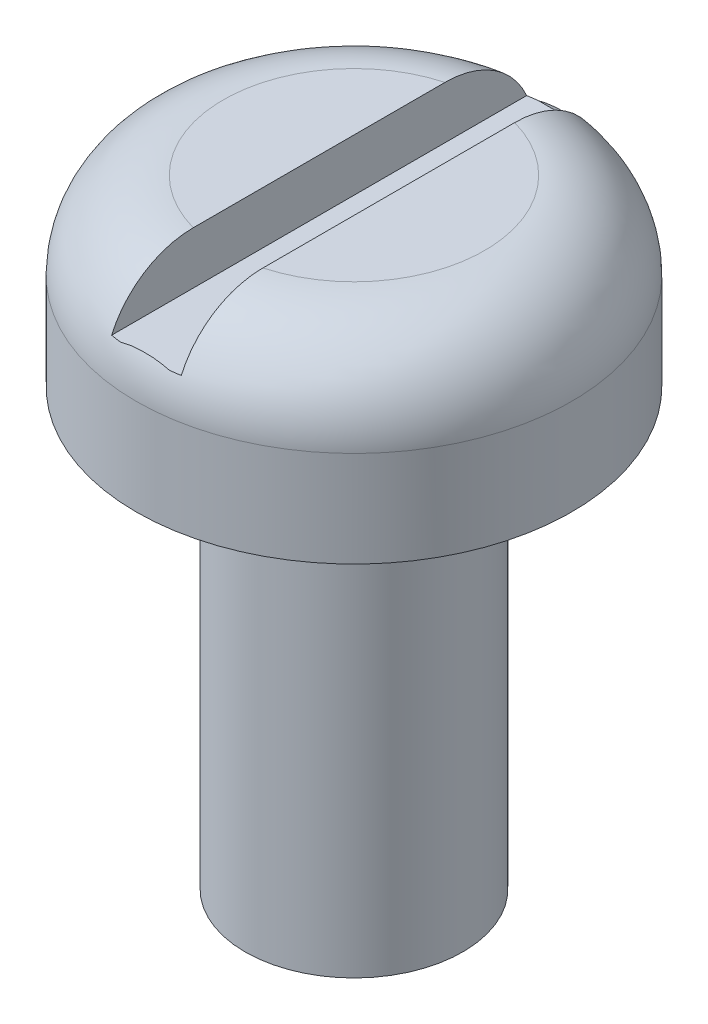
ISO-10303-21;
HEADER;
FILE_DESCRIPTION(('STEP AP214'),'2;1');
FILE_NAME('part.step','',(''),(''),'','','');
FILE_SCHEMA(('AUTOMOTIVE_DESIGN { 1 0 10303 214 1 1 1 1 }'));
ENDSEC;
DATA;
#1=APPLICATION_CONTEXT('core data for automotive mechanical design processes');
#2=APPLICATION_PROTOCOL_DEFINITION('international standard','automotive_design',2000,#1);
#3=PRODUCT_CONTEXT('',#1,'mechanical');
#4=PRODUCT('Part','Part','',(#3));
#5=PRODUCT_RELATED_PRODUCT_CATEGORY('part','',(#4));
#6=PRODUCT_DEFINITION_FORMATION('','',#4);
#7=PRODUCT_DEFINITION_CONTEXT('part definition',#1,'design');
#8=PRODUCT_DEFINITION('design','',#6,#7);
#9=PRODUCT_DEFINITION_SHAPE('','',#8);
#10=(LENGTH_UNIT() NAMED_UNIT(*) SI_UNIT(.MILLI.,.METRE.));
#11=(NAMED_UNIT(*) PLANE_ANGLE_UNIT() SI_UNIT($,.RADIAN.));
#12=(NAMED_UNIT(*) SI_UNIT($,.STERADIAN.) SOLID_ANGLE_UNIT());
#13=UNCERTAINTY_MEASURE_WITH_UNIT(LENGTH_MEASURE(1.E-05),#10,'distance_accuracy_value','');
#14=(GEOMETRIC_REPRESENTATION_CONTEXT(3) GLOBAL_UNCERTAINTY_ASSIGNED_CONTEXT((#13)) GLOBAL_UNIT_ASSIGNED_CONTEXT((#10,
#11,#12)) REPRESENTATION_CONTEXT('',''));
#15=CARTESIAN_POINT('',(0.,0.,0.));
#16=DIRECTION('',(0.,0.,1.));
#17=DIRECTION('',(1.,0.,0.));
#18=AXIS2_PLACEMENT_3D('',#15,#16,#17);
#19=CARTESIAN_POINT('',(0.,2.1,0.));
#20=DIRECTION('',(0.,-1.,0.));
#21=DIRECTION('',(0.,0.,-1.));
#22=AXIS2_PLACEMENT_3D('',#19,#20,#21);
#23=PLANE('',#22);
#24=CARTESIAN_POINT('',(0.,2.1,0.));
#25=DIRECTION('',(0.,-1.,0.));
#26=DIRECTION('',(0.,0.,-1.));
#27=AXIS2_PLACEMENT_3D('',#24,#25,#26);
#28=CIRCLE('',#27,1.5);
#29=CARTESIAN_POINT('',(0.4,2.1,1.4456832294801));
#30=VERTEX_POINT('',#29);
#31=CARTESIAN_POINT('',(0.4,2.1,-1.4456832294801));
#32=VERTEX_POINT('',#31);
#33=EDGE_CURVE('E110',#30,#32,#28,.F.);
#34=ORIENTED_EDGE('',*,*,#33,.T.);
#35=DIRECTION('',(0.,0.,-1.));
#36=VECTOR('',#35,1.);
#37=CARTESIAN_POINT('',(0.4,2.1,2.4));
#38=LINE('',#37,#36);
#39=EDGE_CURVE('E97',#30,#32,#38,.T.);
#40=ORIENTED_EDGE('',*,*,#39,.F.);
#41=EDGE_LOOP('',(#34,#40));
#42=FACE_BOUND('',#41,.T.);
#43=ADVANCED_FACE('F39',(#42),#23,.F.);
#44=CARTESIAN_POINT('',(0.,-5.,0.));
#45=DIRECTION('',(0.,1.,0.));
#46=DIRECTION('',(0.,0.,1.));
#47=AXIS2_PLACEMENT_3D('',#44,#45,#46);
#48=PLANE('',#47);
#49=CARTESIAN_POINT('',(0.,-5.,0.));
#50=DIRECTION('',(0.,1.,0.));
#51=DIRECTION('',(0.,0.,1.));
#52=AXIS2_PLACEMENT_3D('',#49,#50,#51);
#53=CIRCLE('',#52,1.25);
#54=CARTESIAN_POINT('',(0.,-5.,1.25));
#55=VERTEX_POINT('',#54);
#56=EDGE_CURVE('E113',#55,#55,#53,.T.);
#57=ORIENTED_EDGE('',*,*,#56,.F.);
#58=EDGE_LOOP('',(#57));
#59=FACE_BOUND('',#58,.T.);
#60=ADVANCED_FACE('F172',(#59),#48,.F.);
#61=CARTESIAN_POINT('',(0.,4.11096256684492,0.));
#62=DIRECTION('',(0.,1.,0.));
#63=DIRECTION('',(0.,0.,1.));
#64=AXIS2_PLACEMENT_3D('',#61,#62,#63);
#65=CYLINDRICAL_SURFACE('',#64,1.25);
#66=CARTESIAN_POINT('',(0.,0.,0.));
#67=DIRECTION('',(0.,1.,0.));
#68=DIRECTION('',(0.,0.,1.));
#69=AXIS2_PLACEMENT_3D('',#66,#67,#68);
#70=CIRCLE('',#69,1.25);
#71=CARTESIAN_POINT('',(0.,0.,1.25));
#72=VERTEX_POINT('',#71);
#73=EDGE_CURVE('E116',#72,#72,#70,.T.);
#74=ORIENTED_EDGE('',*,*,#73,.F.);
#75=EDGE_LOOP('',(#74));
#76=FACE_BOUND('',#75,.T.);
#77=ORIENTED_EDGE('',*,*,#56,.T.);
#78=EDGE_LOOP('',(#77));
#79=FACE_BOUND('',#78,.T.);
#80=ADVANCED_FACE('F180',(#76,#79),#65,.T.);
#81=CARTESIAN_POINT('',(1.25,0.,0.));
#82=DIRECTION('',(0.,1.,0.));
#83=DIRECTION('',(0.,0.,1.));
#84=AXIS2_PLACEMENT_3D('',#81,#82,#83);
#85=PLANE('',#84);
#86=CARTESIAN_POINT('',(0.,0.,0.));
#87=DIRECTION('',(0.,1.,0.));
#88=DIRECTION('',(0.,0.,1.));
#89=AXIS2_PLACEMENT_3D('',#86,#87,#88);
#90=CIRCLE('',#89,2.5);
#91=CARTESIAN_POINT('',(0.,0.,2.5));
#92=VERTEX_POINT('',#91);
#93=EDGE_CURVE('E201',#92,#92,#90,.T.);
#94=ORIENTED_EDGE('',*,*,#93,.F.);
#95=EDGE_LOOP('',(#94));
#96=FACE_BOUND('',#95,.T.);
#97=ORIENTED_EDGE('',*,*,#73,.T.);
#98=EDGE_LOOP('',(#97));
#99=FACE_BOUND('',#98,.T.);
#100=ADVANCED_FACE('F188',(#96,#99),#85,.F.);
#101=CARTESIAN_POINT('',(0.,4.11096256684492,0.));
#102=DIRECTION('',(0.,1.,0.));
#103=DIRECTION('',(0.,0.,1.));
#104=AXIS2_PLACEMENT_3D('',#101,#102,#103);
#105=CYLINDRICAL_SURFACE('',#104,2.5);
#106=CARTESIAN_POINT('',(0.,1.1,0.));
#107=DIRECTION('',(0.,-1.,0.));
#108=DIRECTION('',(0.,0.,-1.));
#109=AXIS2_PLACEMENT_3D('',#106,#107,#108);
#110=CIRCLE('',#109,2.5);
#111=CARTESIAN_POINT('',(0.,1.1,-2.5));
#112=VERTEX_POINT('',#111);
#113=EDGE_CURVE('E117',#112,#112,#110,.T.);
#114=ORIENTED_EDGE('',*,*,#113,.T.);
#115=EDGE_LOOP('',(#114));
#116=FACE_BOUND('',#115,.T.);
#117=ORIENTED_EDGE('',*,*,#93,.T.);
#118=EDGE_LOOP('',(#117));
#119=FACE_BOUND('',#118,.T.);
#120=ADVANCED_FACE('F182',(#116,#119),#105,.T.);
#121=CARTESIAN_POINT('',(-0.4,2.1,-1.4456832294801));
#122=VERTEX_POINT('',#121);
#123=CARTESIAN_POINT('',(-0.4,2.1,1.4456832294801));
#124=VERTEX_POINT('',#123);
#125=EDGE_CURVE('E111',#122,#124,#28,.F.);
#126=ORIENTED_EDGE('',*,*,#125,.T.);
#127=DIRECTION('',(0.,0.,1.));
#128=VECTOR('',#127,1.);
#129=CARTESIAN_POINT('',(-0.4,2.1,2.4));
#130=LINE('',#129,#128);
#131=EDGE_CURVE('E107',#122,#124,#130,.T.);
#132=ORIENTED_EDGE('',*,*,#131,.F.);
#133=EDGE_LOOP('',(#126,#132));
#134=FACE_BOUND('',#133,.T.);
#135=ADVANCED_FACE('F147',(#134),#23,.F.);
#136=CARTESIAN_POINT('',(0.,1.1,0.));
#137=DIRECTION('',(0.,-1.,0.));
#138=DIRECTION('',(0.,0.,-1.));
#139=AXIS2_PLACEMENT_3D('',#136,#137,#138);
#140=TOROIDAL_SURFACE('',#139,1.5,1.);
#141=CARTESIAN_POINT('',(-0.4,1.37314136652749,0.359822287950911));
#142=CARTESIAN_POINT('',(-0.4,1.40093270642667,0.371622303440927));
#143=CARTESIAN_POINT('',(-0.4,1.42812821348821,0.384783955279465));
#144=CARTESIAN_POINT('',(-0.4,1.48131846126341,0.413357432969681));
#145=CARTESIAN_POINT('',(-0.4,1.50731251310842,0.428770529152034));
#146=CARTESIAN_POINT('',(-0.4,1.58346389369532,0.477895994599856));
#147=CARTESIAN_POINT('',(-0.4,1.63178371791217,0.514491510849547));
#148=CARTESIAN_POINT('',(-0.4,1.72575940533382,0.596458724839461));
#149=CARTESIAN_POINT('',(-0.4,1.77105848354616,0.642236723330395));
#150=CARTESIAN_POINT('',(-0.4,1.85432920614574,0.739995997687899));
#151=CARTESIAN_POINT('',(-0.4,1.89230615268545,0.791972740397109));
#152=CARTESIAN_POINT('',(-0.4,1.96395225809638,0.908108851081128));
#153=CARTESIAN_POINT('',(-0.4,1.99648409188238,0.972978581679796));
#154=CARTESIAN_POINT('',(-0.4,2.04899259975919,1.10766848251091));
#155=CARTESIAN_POINT('',(-0.4,2.06896827937325,1.17748904437354));
#156=CARTESIAN_POINT('',(-0.4,2.0938680591257,1.31338506858809));
#157=CARTESIAN_POINT('',(-0.4,2.09996775846476,1.37924512842784));
#158=CARTESIAN_POINT('',(-0.4,2.10003193371477,1.51096708389506));
#159=CARTESIAN_POINT('',(-0.4,2.09400361962018,1.57682895516902));
#160=CARTESIAN_POINT('',(-0.4,2.07067030458484,1.70123764081731));
#161=CARTESIAN_POINT('',(-0.4,2.05427474028281,1.75995595824222));
#162=CARTESIAN_POINT('',(-0.4,2.01140744039179,1.8735942289021));
#163=CARTESIAN_POINT('',(-0.4,1.98493845444247,1.92851521382656));
#164=CARTESIAN_POINT('',(-0.4,1.92400229725042,2.03046814640842));
#165=CARTESIAN_POINT('',(-0.4,1.88993659917133,2.07774038262831));
#166=CARTESIAN_POINT('',(-0.4,1.81417105020338,2.16571110461842));
#167=CARTESIAN_POINT('',(-0.4,1.77247236837605,2.20641059527067));
#168=CARTESIAN_POINT('',(-0.4,1.68373611156411,2.27906555988676));
#169=CARTESIAN_POINT('',(-0.4,1.63685221089368,2.31120885230998));
#170=CARTESIAN_POINT('',(-0.4,1.53829665012664,2.36704528781166));
#171=CARTESIAN_POINT('',(-0.4,1.48662538258074,2.39073912295086));
#172=CARTESIAN_POINT('',(-0.4,1.38069618244624,2.4287008656164));
#173=CARTESIAN_POINT('',(-0.4,1.32648106473839,2.44308832578949));
#174=CARTESIAN_POINT('',(-0.4,1.21639976672113,2.4624969216675));
#175=CARTESIAN_POINT('',(-0.4,1.16053365428317,2.46751844185828));
#176=CARTESIAN_POINT('',(-0.4,1.04908863796257,2.46804320743455));
#177=CARTESIAN_POINT('',(-0.4,0.993509988965319,2.46360255553827));
#178=CARTESIAN_POINT('',(-0.4,0.883889082008193,2.4454495710633));
#179=CARTESIAN_POINT('',(-0.4,0.829846804146247,2.43173735864504));
#180=CARTESIAN_POINT('',(-0.4,0.724842061024363,2.39545342961124));
#181=CARTESIAN_POINT('',(-0.4,0.673878716366111,2.37288425663857));
#182=CARTESIAN_POINT('',(-0.4,0.576438813198237,2.31955230734661));
#183=CARTESIAN_POINT('',(-0.4,0.529962302699139,2.28878944336552));
#184=CARTESIAN_POINT('',(-0.4,0.442543206150293,2.2197899814353));
#185=CARTESIAN_POINT('',(-0.4,0.401630600296936,2.18151541483789));
#186=CARTESIAN_POINT('',(-0.4,0.32672353206193,2.0987119502436));
#187=CARTESIAN_POINT('',(-0.4,0.292729339220681,2.05418280868355));
#188=CARTESIAN_POINT('',(-0.4,0.232169698703393,1.95958819897401));
#189=CARTESIAN_POINT('',(-0.4,0.205696783523953,1.90946352616052));
#190=CARTESIAN_POINT('',(-0.4,0.161349431874205,1.80555086102151));
#191=CARTESIAN_POINT('',(-0.4,0.143475492699256,1.75176265703223));
#192=CARTESIAN_POINT('',(-0.4,0.11638434181792,1.64084211977878));
#193=CARTESIAN_POINT('',(-0.4,0.107358832247017,1.58366304903687));
#194=CARTESIAN_POINT('',(-0.4,0.0986849300413458,1.46860383693886));
#195=CARTESIAN_POINT('',(-0.4,0.0990380349972624,1.41072358509211));
#196=CARTESIAN_POINT('',(-0.4,0.109055349478419,1.29367665174019));
#197=CARTESIAN_POINT('',(-0.4,0.119055025193746,1.23453889656783));
#198=CARTESIAN_POINT('',(-0.4,0.148276458995809,1.11861077758735));
#199=CARTESIAN_POINT('',(-0.4,0.167498607758144,1.06182051333261));
#200=CARTESIAN_POINT('',(-0.4,0.215744233840994,0.948547956472629));
#201=CARTESIAN_POINT('',(-0.4,0.245283691181516,0.892285842264092));
#202=CARTESIAN_POINT('',(-0.4,0.3126427582318,0.784941269175456));
#203=CARTESIAN_POINT('',(-0.4,0.350469724634658,0.733863471656097));
#204=CARTESIAN_POINT('',(-0.4,0.436996253406748,0.633386518111079));
#205=CARTESIAN_POINT('',(-0.4,0.486373171812133,0.584566395985288));
#206=CARTESIAN_POINT('',(-0.4,0.565722481216896,0.517693556759759));
#207=CARTESIAN_POINT('',(-0.4,0.593069815311135,0.496451989280449));
#208=CARTESIAN_POINT('',(-0.4,0.649432632497327,0.456320362883837));
#209=CARTESIAN_POINT('',(-0.4,0.678447348158725,0.437429234624265));
#210=CARTESIAN_POINT('',(-0.4,0.745585160405143,0.397942522412036));
#211=CARTESIAN_POINT('',(-0.4,0.784165027026359,0.378111384529633));
#212=CARTESIAN_POINT('',(-0.4,0.86367896280017,0.344038828478993));
#213=CARTESIAN_POINT('',(-0.4,0.904606064923999,0.329781759484785));
#214=CARTESIAN_POINT('',(-0.4,0.980825865665075,0.310823745651696));
#215=CARTESIAN_POINT('',(-0.4,1.01579220394159,0.304857656892121));
#216=CARTESIAN_POINT('',(-0.4,1.08620228902251,0.299138358795534));
#217=CARTESIAN_POINT('',(-0.4,1.12164512863084,0.299374661447218));
#218=CARTESIAN_POINT('',(-0.4,1.19399937284863,0.306183841661282));
#219=CARTESIAN_POINT('',(-0.4,1.23087368500297,0.313130592971764));
#220=CARTESIAN_POINT('',(-0.4,1.30318937641905,0.332611747138802));
#221=CARTESIAN_POINT('',(-0.4,1.33862491613106,0.345166835899453));
#222=CARTESIAN_POINT('',(-0.4,1.37314136652749,0.359822287950911));
#223=B_SPLINE_CURVE_WITH_KNOTS('',3,(#141,#142,#143,#144,#145,#146,#147,#148,#149,#150,#151,
#152,#153,#154,#155,#156,#157,#158,#159,#160,#161,#162,#163,#164,#165,#166,#167,#168,#169,#170,
#171,#172,#173,#174,#175,#176,#177,#178,#179,#180,#181,#182,#183,#184,#185,#186,#187,#188,#189,
#190,#191,#192,#193,#194,#195,#196,#197,#198,#199,#200,#201,#202,#203,#204,#205,#206,#207,#208,
#209,#210,#211,#212,#213,#214,#215,#216,#217,#218,#219,#220,#221,#222),.UNSPECIFIED.,.T.,.F.,(4,
2,2,2,2,2,2,2,2,2,2,2,2,2,2,2,2,2,2,2,2,2,2,2,2,2,2,2,2,2,2,2,2,2,2,2,2,2,2,2,4),(0.,
0.0905235289434078,0.181098332620318,0.362269841007183,0.554796553029223,0.747183323320209,
0.963694489865064,1.18022280244035,1.37758856742685,1.57483703491976,1.75681028240803,
1.93873389409044,2.11268266628051,2.28660481887703,2.45631680998708,2.62601489748268,
2.79348725921426,2.96095274580354,3.12742806687218,3.29390123044403,3.46032661930264,
3.6267537887674,3.79404491531046,3.96134255824518,4.13061715773694,4.29990154552868,
4.47277739199613,4.64568084369387,4.82482230181395,5.00397134926242,5.19380008899763,
5.38379802447056,5.59114286201002,5.69493236376326,5.79867447202674,5.92848389712762,
6.05792618089144,6.16386383384293,6.26962236175429,6.38163469773545,6.49406363811112),.UNSPECIFIED.);
#224=CARTESIAN_POINT('',(-0.4,1.5,2.38317968625396));
#225=VERTEX_POINT('',#224);
#226=EDGE_CURVE('E11',#124,#225,#223,.T.);
#227=ORIENTED_EDGE('',*,*,#226,.F.);
#228=ORIENTED_EDGE('',*,*,#125,.F.);
#229=CARTESIAN_POINT('',(-0.4,1.8398346166564,-2.13565237677622));
#230=CARTESIAN_POINT('',(-0.4,1.87811511422596,-2.09282132200416));
#231=CARTESIAN_POINT('',(-0.4,1.91273739539628,-2.04667706943084));
#232=CARTESIAN_POINT('',(-0.4,1.9736981507183,-1.94917085805161));
#233=CARTESIAN_POINT('',(-0.4,2.00002839113024,-1.89780377965601));
#234=CARTESIAN_POINT('',(-0.4,2.04370446904179,-1.79147021841471));
#235=CARTESIAN_POINT('',(-0.4,2.06106288392302,-1.73650889676743));
#236=CARTESIAN_POINT('',(-0.4,2.08651421395001,-1.62450370159404));
#237=CARTESIAN_POINT('',(-0.4,2.09460879653804,-1.56746020475677));
#238=CARTESIAN_POINT('',(-0.4,2.1015923534082,-1.45156026807819));
#239=CARTESIAN_POINT('',(-0.4,2.10027504131188,-1.39269154127577));
#240=CARTESIAN_POINT('',(-0.4,2.08823795927848,-1.27592889657369));
#241=CARTESIAN_POINT('',(-0.4,2.07751600879707,-1.21803520791779));
#242=CARTESIAN_POINT('',(-0.4,2.04651192813994,-1.10189643658627));
#243=CARTESIAN_POINT('',(-0.4,2.02579623873071,-1.04376749234396));
#244=CARTESIAN_POINT('',(-0.4,1.97558791307315,-0.931458751239951));
#245=CARTESIAN_POINT('',(-0.4,1.94609445975426,-0.877279322600243));
#246=CARTESIAN_POINT('',(-0.4,1.87684180091612,-0.769927471924329));
#247=CARTESIAN_POINT('',(-0.4,1.83646755612036,-0.717152910320781));
#248=CARTESIAN_POINT('',(-0.4,1.74810211866065,-0.618315015681679));
#249=CARTESIAN_POINT('',(-0.4,1.70010141960916,-0.572260198110461));
#250=CARTESIAN_POINT('',(-0.4,1.60407374661698,-0.493257701191677));
#251=CARTESIAN_POINT('',(-0.4,1.55679813188248,-0.459391493969736));
#252=CARTESIAN_POINT('',(-0.4,1.45772774140027,-0.398988471741608));
#253=CARTESIAN_POINT('',(-0.4,1.40594040681274,-0.3724398781033));
#254=CARTESIAN_POINT('',(-0.4,1.31712766928422,-0.337404860189235));
#255=CARTESIAN_POINT('',(-0.4,1.28133192978793,-0.32585030021374));
#256=CARTESIAN_POINT('',(-0.4,1.20841501879743,-0.308692363113694));
#257=CARTESIAN_POINT('',(-0.4,1.17129977255923,-0.303065181631446));
#258=CARTESIAN_POINT('',(-0.4,1.09639434023588,-0.298842814199439));
#259=CARTESIAN_POINT('',(-0.4,1.05860130092844,-0.300294884677492));
#260=CARTESIAN_POINT('',(-0.4,0.983842842535524,-0.31000817938353));
#261=CARTESIAN_POINT('',(-0.4,0.946880436012452,-0.318291032815124));
#262=CARTESIAN_POINT('',(-0.4,0.860704609557469,-0.344400859657943));
#263=CARTESIAN_POINT('',(-0.4,0.812255942900869,-0.364675108716839));
#264=CARTESIAN_POINT('',(-0.4,0.718903552720742,-0.412218542714998));
#265=CARTESIAN_POINT('',(-0.4,0.674011509182348,-0.43950961881602));
#266=CARTESIAN_POINT('',(-0.4,0.571517655577868,-0.511011072420971));
#267=CARTESIAN_POINT('',(-0.4,0.515631483609865,-0.55769855236453));
#268=CARTESIAN_POINT('',(-0.4,0.412373327343274,-0.659567127037799));
#269=CARTESIAN_POINT('',(-0.4,0.364993216969837,-0.714740020827664));
#270=CARTESIAN_POINT('',(-0.4,0.280370897765796,-0.83245480697802));
#271=CARTESIAN_POINT('',(-0.4,0.243130991913634,-0.894998368703986));
#272=CARTESIAN_POINT('',(-0.4,0.180632877755621,-1.0258349342455));
#273=CARTESIAN_POINT('',(-0.4,0.15537019622706,-1.09412578034179));
#274=CARTESIAN_POINT('',(-0.4,0.119675701746921,-1.22925293613442));
#275=CARTESIAN_POINT('',(-0.4,0.1083094069144,-1.29584172967598));
#276=CARTESIAN_POINT('',(-0.4,0.0980372944435982,-1.4299812506074));
#277=CARTESIAN_POINT('',(-0.4,0.0991256650483317,-1.49753151464729));
#278=CARTESIAN_POINT('',(-0.4,0.1134388617548,-1.62553044027083));
#279=CARTESIAN_POINT('',(-0.4,0.125627901028848,-1.68609598851655));
#280=CARTESIAN_POINT('',(-0.4,0.160537119905299,-1.80411252286452));
#281=CARTESIAN_POINT('',(-0.4,0.18325366557044,-1.86156457606121));
#282=CARTESIAN_POINT('',(-0.4,0.237265423673911,-1.96872091375427));
#283=CARTESIAN_POINT('',(-0.4,0.268079596437864,-2.01866808035782));
#284=CARTESIAN_POINT('',(-0.4,0.337877354698562,-2.1124864266054));
#285=CARTESIAN_POINT('',(-0.4,0.376859568393178,-2.15635862447296));
#286=CARTESIAN_POINT('',(-0.4,0.460707820258591,-2.23553974299801));
#287=CARTESIAN_POINT('',(-0.4,0.505383952831932,-2.27104991609509));
#288=CARTESIAN_POINT('',(-0.4,0.600138773125368,-2.33392989072807));
#289=CARTESIAN_POINT('',(-0.4,0.650216959142549,-2.3613004473261));
#290=CARTESIAN_POINT('',(-0.4,0.753540285983831,-2.40671720097111));
#291=CARTESIAN_POINT('',(-0.4,0.80672684064377,-2.42489676658019));
#292=CARTESIAN_POINT('',(-0.4,0.915407372887323,-2.45199540717226));
#293=CARTESIAN_POINT('',(-0.4,0.97090118110374,-2.46091516064094));
#294=CARTESIAN_POINT('',(-0.4,1.08218935346109,-2.46919646455202));
#295=CARTESIAN_POINT('',(-0.4,1.13797858856519,-2.46862712518596));
#296=CARTESIAN_POINT('',(-0.4,1.2486765298021,-2.45811473647918));
#297=CARTESIAN_POINT('',(-0.4,1.30358510001758,-2.44817025411837));
#298=CARTESIAN_POINT('',(-0.4,1.41089189336081,-2.41922009359857));
#299=CARTESIAN_POINT('',(-0.4,1.46329268744568,-2.40022392408609));
#300=CARTESIAN_POINT('',(-0.4,1.56414449701011,-2.35374341893508));
#301=CARTESIAN_POINT('',(-0.4,1.61259882783671,-2.32626630290257));
#302=CARTESIAN_POINT('',(-0.4,1.69172346832536,-2.27220645824847));
#303=CARTESIAN_POINT('',(-0.4,1.72364016088598,-2.24742317275596));
#304=CARTESIAN_POINT('',(-0.4,1.78425113542326,-2.19418900505821));
#305=CARTESIAN_POINT('',(-0.4,1.81294536457515,-2.1657380627467));
#306=CARTESIAN_POINT('',(-0.4,1.8398346166564,-2.13565237677622));
#307=B_SPLINE_CURVE_WITH_KNOTS('',3,(#229,#230,#231,#232,#233,#234,#235,#236,#237,#238,#239,
#240,#241,#242,#243,#244,#245,#246,#247,#248,#249,#250,#251,#252,#253,#254,#255,#256,#257,#258,
#259,#260,#261,#262,#263,#264,#265,#266,#267,#268,#269,#270,#271,#272,#273,#274,#275,#276,#277,
#278,#279,#280,#281,#282,#283,#284,#285,#286,#287,#288,#289,#290,#291,#292,#293,#294,#295,#296,
#297,#298,#299,#300,#301,#302,#303,#304,#305,#306),.UNSPECIFIED.,.T.,.F.,(4,2,2,2,2,2,2,2,2,2,2,
2,2,2,2,2,2,2,2,2,2,2,2,2,2,2,2,2,2,2,2,2,2,2,2,2,2,2,4),(0.,0.172184298385887,
0.344539035262126,0.516651492411426,0.688732965326791,0.864597445019219,1.04050271114878,
1.22483852285103,1.40919149866263,1.60772172388315,1.80650138740882,1.98046561411988,
2.15414816588351,2.26662084266058,2.37864008660523,2.49140811714806,2.60453459710285,
2.76123319410837,2.91842672169672,3.13581311127636,3.35299070753946,3.57021758672807,
3.78736327255022,3.98892059797868,4.19038387395919,4.3747828674368,4.55911825650523,
4.73431654184073,4.90948542661124,5.07986730131038,5.25023336579799,5.41805071955777,
5.58585577612322,5.75243922600576,5.91904814282181,6.08548242430151,6.25177541361406,
6.37272031802962,6.49366720476529),.UNSPECIFIED.);
#308=CARTESIAN_POINT('',(-0.4,1.5,-2.38317968625396));
#309=VERTEX_POINT('',#308);
#310=EDGE_CURVE('E161',#309,#122,#307,.T.);
#311=ORIENTED_EDGE('',*,*,#310,.F.);
#312=CARTESIAN_POINT('',(0.,1.5,0.));
#313=DIRECTION('',(0.,-1.,0.));
#314=DIRECTION('',(0.,0.,-1.));
#315=AXIS2_PLACEMENT_3D('',#312,#313,#314);
#316=CIRCLE('',#315,2.41651513899117);
#317=CARTESIAN_POINT('',(-0.28203797080093,1.5,-2.4));
#318=VERTEX_POINT('',#317);
#319=EDGE_CURVE('E126',#318,#309,#316,.F.);
#320=ORIENTED_EDGE('',*,*,#319,.F.);
#321=CARTESIAN_POINT('',(0.,1.53588989435483,-2.4));
#322=CARTESIAN_POINT('',(-0.0523613978899214,1.53588901877393,-2.4));
#323=CARTESIAN_POINT('',(-0.104706301254776,1.5323813334837,-2.4));
#324=CARTESIAN_POINT('',(-0.208501891004427,1.51799953053408,-2.4));
#325=CARTESIAN_POINT('',(-0.259951628531131,1.50711803303479,-2.4));
#326=CARTESIAN_POINT('',(-0.346409581768874,1.48111211180436,-2.4));
#327=CARTESIAN_POINT('',(-0.382021879902106,1.46800005995611,-2.4));
#328=CARTESIAN_POINT('',(-0.450941398840353,1.43669713505295,-2.4));
#329=CARTESIAN_POINT('',(-0.484253992751854,1.41851863768282,-2.4));
#330=CARTESIAN_POINT('',(-0.53598493066441,1.3836324587465,-2.4));
#331=CARTESIAN_POINT('',(-0.555545154950903,1.36862388379171,-2.4));
#332=CARTESIAN_POINT('',(-0.592248046819968,1.33587444818732,-2.4));
#333=CARTESIAN_POINT('',(-0.609393974054034,1.31813734053445,-2.4));
#334=CARTESIAN_POINT('',(-0.636766968840443,1.28417421975245,-2.4));
#335=CARTESIAN_POINT('',(-0.647682643300757,1.26850715509958,-2.4));
#336=CARTESIAN_POINT('',(-0.666844871892905,1.2356021442328,-2.4));
#337=CARTESIAN_POINT('',(-0.675093129713662,1.21836520975417,-2.4));
#338=CARTESIAN_POINT('',(-0.688361963068741,1.18247001515464,-2.4));
#339=CARTESIAN_POINT('',(-0.693349446725192,1.16379926857149,-2.4));
#340=CARTESIAN_POINT('',(-0.699456124075725,1.12583686204735,-2.4));
#341=CARTESIAN_POINT('',(-0.700579314315966,1.10654586444603,-2.4));
#342=CARTESIAN_POINT('',(-0.698982388564146,1.07111275085064,-2.4));
#343=CARTESIAN_POINT('',(-0.696826334423357,1.05494228058384,-2.4));
#344=CARTESIAN_POINT('',(-0.689842968651001,1.02319299167532,-2.4));
#345=CARTESIAN_POINT('',(-0.685015214160056,1.00761427157935,-2.4));
#346=CARTESIAN_POINT('',(-0.672971317357541,0.977285040444597,-2.4));
#347=CARTESIAN_POINT('',(-0.665737208056643,0.96254176693789,-2.4));
#348=CARTESIAN_POINT('',(-0.649292920581298,0.93421328325161,-2.4));
#349=CARTESIAN_POINT('',(-0.640081924470275,0.920628555681094,-2.4));
#350=CARTESIAN_POINT('',(-0.614131667104711,0.887009146193266,-2.4));
#351=CARTESIAN_POINT('',(-0.59616496628996,0.867920387594308,-2.4));
#352=CARTESIAN_POINT('',(-0.557444114576843,0.832811320631153,-2.4));
#353=CARTESIAN_POINT('',(-0.536682298578189,0.81679975488229,-2.4));
#354=CARTESIAN_POINT('',(-0.48175423735787,0.779855337276982,-2.4));
#355=CARTESIAN_POINT('',(-0.446319188230609,0.760816822377176,-2.4));
#356=CARTESIAN_POINT('',(-0.373003467231174,0.728370901201647,-2.4));
#357=CARTESIAN_POINT('',(-0.335118586354998,0.714973500184752,-2.4));
#358=CARTESIAN_POINT('',(-0.238763921722061,0.687566388421427,-2.4));
#359=CARTESIAN_POINT('',(-0.179435892198526,0.676572450972253,-2.4));
#360=CARTESIAN_POINT('',(-0.0597018671642062,0.664048254406671,-2.4));
#361=CARTESIAN_POINT('',(0.000706771866009743,0.662545745289735,-2.4));
#362=CARTESIAN_POINT('',(0.122605782874481,0.66895138836452,-2.4));
#363=CARTESIAN_POINT('',(0.184083615498998,0.677104439841001,-2.4));
#364=CARTESIAN_POINT('',(0.30449967653764,0.704300457485726,-2.4));
#365=CARTESIAN_POINT('',(0.363449533491167,0.723286084239843,-2.4));
#366=CARTESIAN_POINT('',(0.444603614122324,0.760560145967767,-2.4));
#367=CARTESIAN_POINT('',(0.46925883149115,0.773541652498196,-2.4));
#368=CARTESIAN_POINT('',(0.5166960820626,0.802613065674209,-2.4));
#369=CARTESIAN_POINT('',(0.53947926303802,0.818701047114247,-2.4));
#370=CARTESIAN_POINT('',(0.578671036544838,0.851351770686174,-2.4));
#371=CARTESIAN_POINT('',(0.595510118866274,0.867392976948132,-2.4));
#372=CARTESIAN_POINT('',(0.62640936575223,0.901974105206407,-2.4));
#373=CARTESIAN_POINT('',(0.640474154024605,0.920509781598291,-2.4));
#374=CARTESIAN_POINT('',(0.661811049261675,0.955101514563963,-2.4));
#375=CARTESIAN_POINT('',(0.669903074796716,0.970649380345786,-2.4));
#376=CARTESIAN_POINT('',(0.683431539268521,1.00286692510141,-2.4));
#377=CARTESIAN_POINT('',(0.688870107731138,1.01953569223239,-2.4));
#378=CARTESIAN_POINT('',(0.696699100774386,1.05369880784836,-2.4));
#379=CARTESIAN_POINT('',(0.6990699010849,1.07119773634513,-2.4));
#380=CARTESIAN_POINT('',(0.700479091575717,1.10632905548939,-2.4));
#381=CARTESIAN_POINT('',(0.699518346466311,1.12396141032037,-2.4));
#382=CARTESIAN_POINT('',(0.694608935877058,1.15706153285889,-2.4));
#383=CARTESIAN_POINT('',(0.690955929040979,1.17257461497621,-2.4));
#384=CARTESIAN_POINT('',(0.681265986657472,1.20283111624506,-2.4));
#385=CARTESIAN_POINT('',(0.675228155889977,1.21757424401379,-2.4));
#386=CARTESIAN_POINT('',(0.658753212008124,1.25080283779591,-2.4));
#387=CARTESIAN_POINT('',(0.647520268471365,1.26889311993647,-2.4));
#388=CARTESIAN_POINT('',(0.622278118696446,1.3030137768156,-2.4));
#389=CARTESIAN_POINT('',(0.608263754242337,1.31904023168795,-2.4));
#390=CARTESIAN_POINT('',(0.571546978560763,1.35564189292264,-2.4));
#391=CARTESIAN_POINT('',(0.547739743098911,1.37510344878727,-2.4));
#392=CARTESIAN_POINT('',(0.49740965677689,1.41010416028124,-2.4));
#393=CARTESIAN_POINT('',(0.470880515970012,1.42563392953936,-2.4));
#394=CARTESIAN_POINT('',(0.400638905338788,1.46101012724825,-2.4));
#395=CARTESIAN_POINT('',(0.355671020951503,1.47835412721587,-2.4));
#396=CARTESIAN_POINT('',(0.263714667351365,1.50595806706949,-2.4));
#397=CARTESIAN_POINT('',(0.216725187081254,1.51621441742404,-2.4));
#398=CARTESIAN_POINT('',(0.113273540437045,1.53179032560624,-2.4));
#399=CARTESIAN_POINT('',(0.0566271244602953,1.5358908412667,-2.4));
#400=CARTESIAN_POINT('',(0.,1.53588989435483,-2.4));
#401=B_SPLINE_CURVE_WITH_KNOTS('',3,(#321,#322,#323,#324,#325,#326,#327,#328,#329,#330,#331,
#332,#333,#334,#335,#336,#337,#338,#339,#340,#341,#342,#343,#344,#345,#346,#347,#348,#349,#350,
#351,#352,#353,#354,#355,#356,#357,#358,#359,#360,#361,#362,#363,#364,#365,#366,#367,#368,#369,
#370,#371,#372,#373,#374,#375,#376,#377,#378,#379,#380,#381,#382,#383,#384,#385,#386,#387,#388,
#389,#390,#391,#392,#393,#394,#395,#396,#397,#398,#399,#400),.UNSPECIFIED.,.T.,.F.,(4,2,2,2,2,2,
2,2,2,2,2,2,2,2,2,2,2,2,2,2,2,2,2,2,2,2,2,2,2,2,2,2,2,2,2,2,2,2,2,4),(0.,0.15694299290988,
0.314043289537583,0.427593851964513,0.54086944210845,0.614629404086063,0.688288804402314,
0.745363419034541,0.802401507569192,0.860009812719194,0.917558520020611,0.966263972079827,
1.01497749994353,1.06406323073925,1.11316931003506,1.19136319533519,1.26977605549766,
1.38978005100671,1.50999600188651,1.69006150098099,1.87065321315338,2.05592520565784,
2.24022548840998,2.32364356094146,2.40701010095913,2.47654632396124,2.54596565835216,
2.5983447730951,2.65068178166906,2.70335195728058,2.75600846325,2.80361054117386,
2.85123050507103,2.91475897156288,2.97840637302633,3.07014091853825,3.16209244005676,
3.30588418295201,3.44974869573433,3.61947736515149),.UNSPECIFIED.);
#402=CARTESIAN_POINT('',(0.28203797080093,1.5,-2.4));
#403=VERTEX_POINT('',#402);
#404=EDGE_CURVE('E68',#403,#318,#401,.T.);
#405=ORIENTED_EDGE('',*,*,#404,.F.);
#406=CARTESIAN_POINT('',(0.4,1.5,-2.38317968625396));
#407=VERTEX_POINT('',#406);
#408=EDGE_CURVE('E127',#407,#403,#316,.F.);
#409=ORIENTED_EDGE('',*,*,#408,.F.);
#410=CARTESIAN_POINT('',(0.4,1.8398346166564,-2.13565237677622));
#411=CARTESIAN_POINT('',(0.4,1.8025336749636,-2.1773814924567));
#412=CARTESIAN_POINT('',(0.4,1.76172527036212,-2.21600449359874));
#413=CARTESIAN_POINT('',(0.4,1.67419408066002,-2.28588631913914));
#414=CARTESIAN_POINT('',(0.4,1.62746769067467,-2.31714062147698));
#415=CARTESIAN_POINT('',(0.4,1.52940876831025,-2.3713390862167));
#416=CARTESIAN_POINT('',(0.4,1.4780756936766,-2.39428226870841));
#417=CARTESIAN_POINT('',(0.4,1.37227586190021,-2.43115925951052));
#418=CARTESIAN_POINT('',(0.4,1.31780951979803,-2.44509425808902));
#419=CARTESIAN_POINT('',(0.4,1.20764488159727,-2.4634832264639));
#420=CARTESIAN_POINT('',(0.4,1.1519562468408,-2.46799509873964));
#421=CARTESIAN_POINT('',(0.4,1.04061458662242,-2.46757599472037));
#422=CARTESIAN_POINT('',(0.4,0.984961560821362,-2.46264510973805));
#423=CARTESIAN_POINT('',(0.4,0.875437139069795,-2.44351552757223));
#424=CARTESIAN_POINT('',(0.4,0.821561107103871,-2.42934334981739));
#425=CARTESIAN_POINT('',(0.4,0.716944678679643,-2.39217700086745));
#426=CARTESIAN_POINT('',(0.4,0.666204283026997,-2.36918282740567));
#427=CARTESIAN_POINT('',(0.4,0.569151411780575,-2.31498074904992));
#428=CARTESIAN_POINT('',(0.4,0.522850481608959,-2.28375217948734));
#429=CARTESIAN_POINT('',(0.4,0.436094862630412,-2.21402518359269));
#430=CARTESIAN_POINT('',(0.4,0.395640302202545,-2.17552659766284));
#431=CARTESIAN_POINT('',(0.4,0.3213414645413,-2.09202200955946));
#432=CARTESIAN_POINT('',(0.4,0.287555852995831,-2.04696383266831));
#433=CARTESIAN_POINT('',(0.4,0.227891359388335,-1.95189008322731));
#434=CARTESIAN_POINT('',(0.4,0.202012924559428,-1.90187423048113));
#435=CARTESIAN_POINT('',(0.4,0.158413534434672,-1.79744939669239));
#436=CARTESIAN_POINT('',(0.4,0.140832303266163,-1.74298213272907));
#437=CARTESIAN_POINT('',(0.4,0.114795654295802,-1.63191605429174));
#438=CARTESIAN_POINT('',(0.4,0.106340922785176,-1.57531707984928));
#439=CARTESIAN_POINT('',(0.4,0.0984860257270242,-1.45990117370177));
#440=CARTESIAN_POINT('',(0.4,0.0993469810992965,-1.40106660969367));
#441=CARTESIAN_POINT('',(0.4,0.110478203390523,-1.28430135517202));
#442=CARTESIAN_POINT('',(0.4,0.120750463073401,-1.2263708587293));
#443=CARTESIAN_POINT('',(0.4,0.150844315521293,-1.11012715318193));
#444=CARTESIAN_POINT('',(0.4,0.17109419842707,-1.05192520481304));
#445=CARTESIAN_POINT('',(0.4,0.220394326481706,-0.939403691266162));
#446=CARTESIAN_POINT('',(0.4,0.249445196684533,-0.885084402176862));
#447=CARTESIAN_POINT('',(0.4,0.317786635283325,-0.777422319402401));
#448=CARTESIAN_POINT('',(0.4,0.357688242728369,-0.724468471340176));
#449=CARTESIAN_POINT('',(0.4,0.445138211573264,-0.625198861237103));
#450=CARTESIAN_POINT('',(0.4,0.49269636471048,-0.578891744902354));
#451=CARTESIAN_POINT('',(0.4,0.588648988874252,-0.498708100347199));
#452=CARTESIAN_POINT('',(0.4,0.636372204048253,-0.464023774067665));
#453=CARTESIAN_POINT('',(0.4,0.736480904238632,-0.402104925619826));
#454=CARTESIAN_POINT('',(0.4,0.78885896045663,-0.374858805869408));
#455=CARTESIAN_POINT('',(0.4,0.878367180985448,-0.338972870676199));
#456=CARTESIAN_POINT('',(0.4,0.914208236578202,-0.327165444507478));
#457=CARTESIAN_POINT('',(0.4,0.987249583485681,-0.309479516815649));
#458=CARTESIAN_POINT('',(0.4,1.02444373313221,-0.30357702408444));
#459=CARTESIAN_POINT('',(0.4,1.09957847021203,-0.298826050225612));
#460=CARTESIAN_POINT('',(0.4,1.13752249249266,-0.300028282927865));
#461=CARTESIAN_POINT('',(0.4,1.21261201956484,-0.309330320871159));
#462=CARTESIAN_POINT('',(0.4,1.24975467798643,-0.317451539171653));
#463=CARTESIAN_POINT('',(0.4,1.33584561607568,-0.343124650310172));
#464=CARTESIAN_POINT('',(0.4,1.38406062441165,-0.363057684544076));
#465=CARTESIAN_POINT('',(0.4,1.47699898380558,-0.409893501643049));
#466=CARTESIAN_POINT('',(0.4,1.52171059414888,-0.436818516224861));
#467=CARTESIAN_POINT('',(0.4,1.62418868863823,-0.507642409987047));
#468=CARTESIAN_POINT('',(0.4,1.68022517811658,-0.554061952942187));
#469=CARTESIAN_POINT('',(0.4,1.78383608414852,-0.655412406612993));
#470=CARTESIAN_POINT('',(0.4,1.83141849358401,-0.710335185019087));
#471=CARTESIAN_POINT('',(0.4,1.91652608064444,-0.827596525276821));
#472=CARTESIAN_POINT('',(0.4,1.95404502335848,-0.889939650100518));
#473=CARTESIAN_POINT('',(0.4,2.01715539708709,-1.02041866419952));
#474=CARTESIAN_POINT('',(0.4,2.04275159582965,-1.08855222505529));
#475=CARTESIAN_POINT('',(0.4,2.07916508971908,-1.22355086157526));
#476=CARTESIAN_POINT('',(0.4,2.09089329611194,-1.29016953787581));
#477=CARTESIAN_POINT('',(0.4,2.10187229808395,-1.4244473621843));
#478=CARTESIAN_POINT('',(0.4,2.10112683765856,-1.4921061918967));
#479=CARTESIAN_POINT('',(0.4,2.08743822937752,-1.62035805386721));
#480=CARTESIAN_POINT('',(0.4,2.07553534121961,-1.6810635368071));
#481=CARTESIAN_POINT('',(0.4,2.04116476146503,-1.79936962775553));
#482=CARTESIAN_POINT('',(0.4,2.01870936405181,-1.85697376216796));
#483=CARTESIAN_POINT('',(0.4,1.97115210287696,-1.95248575184529));
#484=CARTESIAN_POINT('',(0.4,1.94834633710307,-1.99155451325902));
#485=CARTESIAN_POINT('',(0.4,1.89773243885747,-2.0663065331936));
#486=CARTESIAN_POINT('',(0.4,1.86992475425431,-2.10199009438652));
#487=CARTESIAN_POINT('',(0.4,1.8398346166564,-2.13565237677622));
#488=B_SPLINE_CURVE_WITH_KNOTS('',3,(#410,#411,#412,#413,#414,#415,#416,#417,#418,#419,#420,
#421,#422,#423,#424,#425,#426,#427,#428,#429,#430,#431,#432,#433,#434,#435,#436,#437,#438,#439,
#440,#441,#442,#443,#444,#445,#446,#447,#448,#449,#450,#451,#452,#453,#454,#455,#456,#457,#458,
#459,#460,#461,#462,#463,#464,#465,#466,#467,#468,#469,#470,#471,#472,#473,#474,#475,#476,#477,
#478,#479,#480,#481,#482,#483,#484,#485,#486,#487),.UNSPECIFIED.,.T.,.F.,(4,2,2,2,2,2,2,2,2,2,2,
2,2,2,2,2,2,2,2,2,2,2,2,2,2,2,2,2,2,2,2,2,2,2,2,2,2,2,4),(0.,0.16775057472048,0.335603829051749,
0.503476867433728,0.6713277199025,0.838144104213449,1.00495887539679,1.17129703809673,
1.33763524353484,1.50439492373876,1.67115826522321,1.8393289332223,2.00750911126255,
2.17842841332394,2.34936056721816,2.52509612406037,2.70086890001929,2.88494730055624,
3.06903877757144,3.26714080909577,3.46549823008536,3.64196959282255,3.81816421084223,
3.93100607293198,4.04338758381886,4.15657224304483,4.27010846692086,4.42577242455246,
4.58193752455996,4.79915529906802,5.01616660008016,5.23331204343933,5.45037057886174,
5.65219992357299,5.8539686898992,6.03861870316791,6.22305412156803,6.35838822907961,
6.49371022488977),.UNSPECIFIED.);
#489=EDGE_CURVE('E114',#32,#407,#488,.T.);
#490=ORIENTED_EDGE('',*,*,#489,.F.);
#491=ORIENTED_EDGE('',*,*,#33,.F.);
#492=CARTESIAN_POINT('',(0.4,1.37314136652749,0.359822287950911));
#493=CARTESIAN_POINT('',(0.4,1.34027333235344,0.34586802441915));
#494=CARTESIAN_POINT('',(0.4,1.30658350606981,0.333819173295089));
#495=CARTESIAN_POINT('',(0.4,1.23783156243017,0.314756136386901));
#496=CARTESIAN_POINT('',(0.4,1.20277342782961,0.30772834266681));
#497=CARTESIAN_POINT('',(0.4,1.1466060965669,0.301450771928168));
#498=CARTESIAN_POINT('',(0.4,1.12571391488336,0.3001876483225));
#499=CARTESIAN_POINT('',(0.4,1.08391117468787,0.299850954545539));
#500=CARTESIAN_POINT('',(0.4,1.06300061563295,0.300777451401812));
#501=CARTESIAN_POINT('',(0.4,1.0004975423084,0.30678929629457));
#502=CARTESIAN_POINT('',(0.4,0.959200058423051,0.315114212979069));
#503=CARTESIAN_POINT('',(0.4,0.869579617183673,0.341137038487327));
#504=CARTESIAN_POINT('',(0.4,0.821778724515694,0.360528286495451));
#505=CARTESIAN_POINT('',(0.4,0.729560069951039,0.406226655615728));
#506=CARTESIAN_POINT('',(0.4,0.685153956924881,0.432556321835831));
#507=CARTESIAN_POINT('',(0.4,0.582728581729174,0.502274025149008));
#508=CARTESIAN_POINT('',(0.4,0.526464710836666,0.548254834256408));
#509=CARTESIAN_POINT('',(0.4,0.422316284250991,0.648747487990962));
#510=CARTESIAN_POINT('',(0.4,0.374423071296478,0.703250406819742));
#511=CARTESIAN_POINT('',(0.4,0.288555811142847,0.819746910578753));
#512=CARTESIAN_POINT('',(0.4,0.250594938933004,0.881750286936168));
#513=CARTESIAN_POINT('',(0.4,0.186503607088216,1.01162408451799));
#514=CARTESIAN_POINT('',(0.4,0.160369267940376,1.07949257306897));
#515=CARTESIAN_POINT('',(0.4,0.122784151786926,1.21428349051904));
#516=CARTESIAN_POINT('',(0.4,0.110464394449882,1.28096281854002));
#517=CARTESIAN_POINT('',(0.4,0.0983352761532404,1.41545727869211));
#518=CARTESIAN_POINT('',(0.4,0.0985199651712363,1.48327185527737));
#519=CARTESIAN_POINT('',(0.4,0.111182750090953,1.61185537314604));
#520=CARTESIAN_POINT('',(0.4,0.122604269214821,1.67272943837964));
#521=CARTESIAN_POINT('',(0.4,0.156057757399696,1.79148952805803));
#522=CARTESIAN_POINT('',(0.4,0.178086031772774,1.84937658520975));
#523=CARTESIAN_POINT('',(0.4,0.230827464371532,1.95742566318693));
#524=CARTESIAN_POINT('',(0.4,0.261044127568545,2.00783046833566));
#525=CARTESIAN_POINT('',(0.4,0.329739823410466,2.10265604304202));
#526=CARTESIAN_POINT('',(0.4,0.368217409918553,2.14707785775508));
#527=CARTESIAN_POINT('',(0.4,0.451152654123434,2.22739087220353));
#528=CARTESIAN_POINT('',(0.4,0.495413353495358,2.26348561906136));
#529=CARTESIAN_POINT('',(0.4,0.589444913277988,2.32759388909336));
#530=CARTESIAN_POINT('',(0.4,0.639215251395408,2.35560817735877));
#531=CARTESIAN_POINT('',(0.4,0.74202437933128,2.40233256109071));
#532=CARTESIAN_POINT('',(0.4,0.795001413764145,2.42117862439152));
#533=CARTESIAN_POINT('',(0.4,0.903380390122657,2.44963424386105));
#534=CARTESIAN_POINT('',(0.4,0.958782211382543,2.45924425910222));
#535=CARTESIAN_POINT('',(0.4,1.06999591299152,2.46890216984732));
#536=CARTESIAN_POINT('',(0.4,1.12580166982899,2.4690207212055));
#537=CARTESIAN_POINT('',(0.4,1.23663736216453,2.45987047391024));
#538=CARTESIAN_POINT('',(0.4,1.29166731245968,2.45060185454614));
#539=CARTESIAN_POINT('',(0.4,1.39930167523626,2.42297544369291));
#540=CARTESIAN_POINT('',(0.4,1.45190979816412,2.40463209890762));
#541=CARTESIAN_POINT('',(0.4,1.55331563100324,2.35940579176124));
#542=CARTESIAN_POINT('',(0.4,1.60211332093479,2.33252278462683));
#543=CARTESIAN_POINT('',(0.4,1.69472428830194,2.27088824660204));
#544=CARTESIAN_POINT('',(0.4,1.73851785245969,2.23610710639278));
#545=CARTESIAN_POINT('',(0.4,1.81971377295093,2.15975236806381));
#546=CARTESIAN_POINT('',(0.4,1.85711592942616,2.11817855761791));
#547=CARTESIAN_POINT('',(0.4,1.92489024631438,2.02898955844508));
#548=CARTESIAN_POINT('',(0.4,1.95518812194968,1.98131794954284));
#549=CARTESIAN_POINT('',(0.4,2.00751327974929,1.88163887094109));
#550=CARTESIAN_POINT('',(0.4,2.02954012851949,1.82963117420906));
#551=CARTESIAN_POINT('',(0.4,2.06517352903974,1.72173791598358));
#552=CARTESIAN_POINT('',(0.4,2.07861616986225,1.66579828763106));
#553=CARTESIAN_POINT('',(0.4,2.09622636803848,1.55248302693321));
#554=CARTESIAN_POINT('',(0.4,2.10039264122771,1.49510719688038));
#555=CARTESIAN_POINT('',(0.4,2.09953576191837,1.37860376576383));
#556=CARTESIAN_POINT('',(0.4,2.09421596067869,1.31947852166978));
#557=CARTESIAN_POINT('',(0.4,2.0742336012562,1.20284897462112));
#558=CARTESIAN_POINT('',(0.4,2.05957080858121,1.14534471238806));
#559=CARTESIAN_POINT('',(0.4,2.02058801304203,1.03031784839436));
#560=CARTESIAN_POINT('',(0.4,1.99579873197548,0.972954781460049));
#561=CARTESIAN_POINT('',(0.4,1.9376497923449,0.862720897423772));
#562=CARTESIAN_POINT('',(0.4,1.90428264283947,0.809854060797754));
#563=CARTESIAN_POINT('',(0.4,1.82700220890959,0.70538239110404));
#564=CARTESIAN_POINT('',(0.4,1.78243566767025,0.654262424734771));
#565=CARTESIAN_POINT('',(0.4,1.68600688067005,0.559506290787704));
#566=CARTESIAN_POINT('',(0.4,1.6341517577829,0.515862907914858));
#567=CARTESIAN_POINT('',(0.4,1.54694664925248,0.453725823116834));
#568=CARTESIAN_POINT('',(0.4,1.51365626661973,0.432302520947485));
#569=CARTESIAN_POINT('',(0.4,1.44496072366373,0.393080461315127));
#570=CARTESIAN_POINT('',(0.4,1.4095553830846,0.37528201336671));
#571=CARTESIAN_POINT('',(0.4,1.37314136652749,0.359822287950911));
#572=B_SPLINE_CURVE_WITH_KNOTS('',3,(#492,#493,#494,#495,#496,#497,#498,#499,#500,#501,#502,
#503,#504,#505,#506,#507,#508,#509,#510,#511,#512,#513,#514,#515,#516,#517,#518,#519,#520,#521,
#522,#523,#524,#525,#526,#527,#528,#529,#530,#531,#532,#533,#534,#535,#536,#537,#538,#539,#540,
#541,#542,#543,#544,#545,#546,#547,#548,#549,#550,#551,#552,#553,#554,#555,#556,#557,#558,#559,
#560,#561,#562,#563,#564,#565,#566,#567,#568,#569,#570,#571),.UNSPECIFIED.,.T.,.F.,(4,2,2,2,2,2,
2,2,2,2,2,2,2,2,2,2,2,2,2,2,2,2,2,2,2,2,2,2,2,2,2,2,2,2,2,2,2,2,2,4),(0.,0.107054780842214,
0.213818312605814,0.276502057784583,0.339187721831683,0.464755421404291,0.618706936564997,
0.773164992539457,0.990074814120148,1.20675895422601,1.42372907946247,1.64062797928978,
1.84294615761334,2.04516806704216,2.23003207061022,2.41483172639059,2.5902696911988,
2.76567696927576,2.9361868665939,3.10668061402622,3.27456234433225,3.44243572974181,
3.60905932387225,3.77567973565159,3.94203574196014,4.10839262048529,4.27538376328065,
4.44238012690651,4.61105170502566,4.77973212014586,4.95154402065011,5.12337970428144,
5.30068361397947,5.47799197386035,5.66466779185065,5.85150718850412,6.05414815970141,
6.25659245640156,6.37518676741234,6.49379120056657),.UNSPECIFIED.);
#573=CARTESIAN_POINT('',(0.4,1.5,2.38317968625396));
#574=VERTEX_POINT('',#573);
#575=EDGE_CURVE('E96',#574,#30,#572,.T.);
#576=ORIENTED_EDGE('',*,*,#575,.F.);
#577=CARTESIAN_POINT('',(0.282037970800937,1.5,2.4));
#578=VERTEX_POINT('',#577);
#579=EDGE_CURVE('E159',#578,#574,#316,.F.);
#580=ORIENTED_EDGE('',*,*,#579,.F.);
#581=CARTESIAN_POINT('',(0.,1.53588989435484,2.4));
#582=CARTESIAN_POINT('',(0.0523613978899219,1.53588901877393,2.4));
#583=CARTESIAN_POINT('',(0.104706301254777,1.53238133348371,2.4));
#584=CARTESIAN_POINT('',(0.208501891004429,1.51799953053408,2.4));
#585=CARTESIAN_POINT('',(0.259951628531133,1.50711803303479,2.4));
#586=CARTESIAN_POINT('',(0.346409581768876,1.48111211180436,2.4));
#587=CARTESIAN_POINT('',(0.382021879902109,1.46800005995611,2.4));
#588=CARTESIAN_POINT('',(0.450941398840355,1.43669713505296,2.4));
#589=CARTESIAN_POINT('',(0.484253992751856,1.41851863768282,2.4));
#590=CARTESIAN_POINT('',(0.535984930664412,1.3836324587465,2.4));
#591=CARTESIAN_POINT('',(0.555545154950904,1.36862388379172,2.4));
#592=CARTESIAN_POINT('',(0.59224804681997,1.33587444818732,2.4));
#593=CARTESIAN_POINT('',(0.609393974054037,1.31813734053445,2.4));
#594=CARTESIAN_POINT('',(0.636766968840446,1.28417421975245,2.4));
#595=CARTESIAN_POINT('',(0.647682643300759,1.26850715509958,2.4));
#596=CARTESIAN_POINT('',(0.666844871892908,1.23560214423281,2.4));
#597=CARTESIAN_POINT('',(0.675093129713665,1.21836520975417,2.4));
#598=CARTESIAN_POINT('',(0.688361963068746,1.18247001515464,2.4));
#599=CARTESIAN_POINT('',(0.693349446725196,1.16379926857149,2.4));
#600=CARTESIAN_POINT('',(0.699456124075729,1.12583686204735,2.4));
#601=CARTESIAN_POINT('',(0.700579314315969,1.10654586444603,2.4));
#602=CARTESIAN_POINT('',(0.698982388564149,1.07111275085064,2.4));
#603=CARTESIAN_POINT('',(0.696826334423361,1.05494228058384,2.4));
#604=CARTESIAN_POINT('',(0.689842968651006,1.02319299167532,2.4));
#605=CARTESIAN_POINT('',(0.685015214160061,1.00761427157935,2.4));
#606=CARTESIAN_POINT('',(0.672971317357547,0.977285040444598,2.4));
#607=CARTESIAN_POINT('',(0.665737208056649,0.962541766937891,2.4));
#608=CARTESIAN_POINT('',(0.649292920581303,0.934213283251612,2.4));
#609=CARTESIAN_POINT('',(0.640081924470279,0.920628555681096,2.4));
#610=CARTESIAN_POINT('',(0.614131667104715,0.887009146193268,2.4));
#611=CARTESIAN_POINT('',(0.596164966289964,0.86792038759431,2.4));
#612=CARTESIAN_POINT('',(0.557444114576848,0.832811320631154,2.4));
#613=CARTESIAN_POINT('',(0.536682298578194,0.816799754882291,2.4));
#614=CARTESIAN_POINT('',(0.481754237357876,0.779855337276983,2.4));
#615=CARTESIAN_POINT('',(0.446319188230615,0.760816822377177,2.4));
#616=CARTESIAN_POINT('',(0.373003467231181,0.728370901201647,2.4));
#617=CARTESIAN_POINT('',(0.335118586355005,0.714973500184752,2.4));
#618=CARTESIAN_POINT('',(0.238763921722069,0.687566388421426,2.4));
#619=CARTESIAN_POINT('',(0.179435892198533,0.676572450972251,2.4));
#620=CARTESIAN_POINT('',(0.0597018671642142,0.664048254406669,2.4));
#621=CARTESIAN_POINT('',(-0.000706771866001741,0.662545745289733,2.4));
#622=CARTESIAN_POINT('',(-0.122605782874473,0.668951388364518,2.4));
#623=CARTESIAN_POINT('',(-0.18408361549899,0.677104439840998,2.4));
#624=CARTESIAN_POINT('',(-0.304499676537632,0.704300457485722,2.4));
#625=CARTESIAN_POINT('',(-0.36344953349116,0.723286084239838,2.4));
#626=CARTESIAN_POINT('',(-0.444603614122317,0.760560145967761,2.4));
#627=CARTESIAN_POINT('',(-0.469258831491144,0.773541652498189,2.4));
#628=CARTESIAN_POINT('',(-0.516696082062595,0.802613065674203,2.4));
#629=CARTESIAN_POINT('',(-0.539479263038015,0.818701047114242,2.4));
#630=CARTESIAN_POINT('',(-0.578671036544835,0.851351770686168,2.4));
#631=CARTESIAN_POINT('',(-0.595510118866272,0.867392976948126,2.4));
#632=CARTESIAN_POINT('',(-0.626409365752229,0.901974105206401,2.4));
#633=CARTESIAN_POINT('',(-0.640474154024604,0.920509781598286,2.4));
#634=CARTESIAN_POINT('',(-0.661811049261675,0.955101514563957,2.4));
#635=CARTESIAN_POINT('',(-0.669903074796717,0.97064938034578,2.4));
#636=CARTESIAN_POINT('',(-0.683431539268522,1.00286692510141,2.4));
#637=CARTESIAN_POINT('',(-0.68887010773114,1.01953569223238,2.4));
#638=CARTESIAN_POINT('',(-0.696699100774388,1.05369880784835,2.4));
#639=CARTESIAN_POINT('',(-0.699069901084903,1.07119773634513,2.4));
#640=CARTESIAN_POINT('',(-0.70047909157572,1.10632905548938,2.4));
#641=CARTESIAN_POINT('',(-0.699518346466315,1.12396141032036,2.4));
#642=CARTESIAN_POINT('',(-0.694608935877061,1.15706153285889,2.4));
#643=CARTESIAN_POINT('',(-0.690955929040982,1.17257461497621,2.4));
#644=CARTESIAN_POINT('',(-0.681265986657475,1.20283111624505,2.4));
#645=CARTESIAN_POINT('',(-0.675228155889981,1.21757424401379,2.4));
#646=CARTESIAN_POINT('',(-0.658753212008128,1.25080283779591,2.4));
#647=CARTESIAN_POINT('',(-0.64752026847137,1.26889311993647,2.4));
#648=CARTESIAN_POINT('',(-0.622278118696451,1.3030137768156,2.4));
#649=CARTESIAN_POINT('',(-0.608263754242343,1.31904023168794,2.4));
#650=CARTESIAN_POINT('',(-0.57154697856077,1.35564189292264,2.4));
#651=CARTESIAN_POINT('',(-0.547739743098918,1.37510344878727,2.4));
#652=CARTESIAN_POINT('',(-0.497409656776898,1.41010416028124,2.4));
#653=CARTESIAN_POINT('',(-0.47088051597002,1.42563392953936,2.4));
#654=CARTESIAN_POINT('',(-0.400638905338798,1.46101012724825,2.4));
#655=CARTESIAN_POINT('',(-0.355671020951513,1.47835412721586,2.4));
#656=CARTESIAN_POINT('',(-0.263714667351377,1.50595806706949,2.4));
#657=CARTESIAN_POINT('',(-0.216725187081267,1.51621441742404,2.4));
#658=CARTESIAN_POINT('',(-0.113273540437055,1.53179032560624,2.4));
#659=CARTESIAN_POINT('',(-0.0566271244602999,1.5358908412667,2.4));
#660=CARTESIAN_POINT('',(0.,1.53588989435484,2.4));
#661=B_SPLINE_CURVE_WITH_KNOTS('',3,(#581,#582,#583,#584,#585,#586,#587,#588,#589,#590,#591,
#592,#593,#594,#595,#596,#597,#598,#599,#600,#601,#602,#603,#604,#605,#606,#607,#608,#609,#610,
#611,#612,#613,#614,#615,#616,#617,#618,#619,#620,#621,#622,#623,#624,#625,#626,#627,#628,#629,
#630,#631,#632,#633,#634,#635,#636,#637,#638,#639,#640,#641,#642,#643,#644,#645,#646,#647,#648,
#649,#650,#651,#652,#653,#654,#655,#656,#657,#658,#659,#660),.UNSPECIFIED.,.T.,.F.,(4,2,2,2,2,2,
2,2,2,2,2,2,2,2,2,2,2,2,2,2,2,2,2,2,2,2,2,2,2,2,2,2,2,2,2,2,2,2,2,4),(0.,0.156942992909881,
0.314043289537585,0.427593851964515,0.540869442108452,0.614629404086065,0.688288804402317,
0.745363419034544,0.802401507569194,0.860009812719196,0.917558520020614,0.966263972079829,
1.01497749994354,1.06406323073925,1.11316931003506,1.19136319533519,1.26977605549766,
1.38978005100671,1.50999600188651,1.69006150098099,1.87065321315338,2.05592520565784,
2.24022548840998,2.32364356094146,2.40701010095914,2.47654632396125,2.54596565835216,
2.59834477309511,2.65068178166907,2.70335195728059,2.75600846325001,2.80361054117387,
2.85123050507104,2.91475897156289,2.97840637302634,3.07014091853826,3.16209244005677,
3.30588418295202,3.44974869573433,3.61947736515151),.UNSPECIFIED.);
#662=CARTESIAN_POINT('',(-0.282037970800937,1.5,2.4));
#663=VERTEX_POINT('',#662);
#664=EDGE_CURVE('E102',#663,#578,#661,.T.);
#665=ORIENTED_EDGE('',*,*,#664,.F.);
#666=EDGE_CURVE('E55',#225,#663,#316,.F.);
#667=ORIENTED_EDGE('',*,*,#666,.F.);
#668=EDGE_LOOP('',(#227,#228,#311,#320,#405,#409,#490,#491,#576,#580,#665,#667));
#669=FACE_BOUND('',#668,.T.);
#670=ORIENTED_EDGE('',*,*,#113,.F.);
#671=EDGE_LOOP('',(#670));
#672=FACE_BOUND('',#671,.T.);
#673=ADVANCED_FACE('F41',(#669,#672),#140,.T.);
#674=CARTESIAN_POINT('',(0.4,1.5,2.4));
#675=DIRECTION('',(1.,0.,0.));
#676=DIRECTION('',(0.,0.,-1.));
#677=AXIS2_PLACEMENT_3D('',#674,#675,#676);
#678=PLANE('',#677);
#679=ORIENTED_EDGE('',*,*,#489,.T.);
#680=DIRECTION('',(0.,0.,-1.));
#681=VECTOR('',#680,1.);
#682=CARTESIAN_POINT('',(0.4,1.5,2.4));
#683=LINE('',#682,#681);
#684=EDGE_CURVE('E56',#574,#407,#683,.T.);
#685=ORIENTED_EDGE('',*,*,#684,.F.);
#686=ORIENTED_EDGE('',*,*,#575,.T.);
#687=ORIENTED_EDGE('',*,*,#39,.T.);
#688=EDGE_LOOP('',(#679,#685,#686,#687));
#689=FACE_BOUND('',#688,.T.);
#690=ADVANCED_FACE('F98',(#689),#678,.F.);
#691=CARTESIAN_POINT('',(-0.4,1.5,2.4));
#692=DIRECTION('',(0.,0.,1.));
#693=DIRECTION('',(1.,0.,0.));
#694=AXIS2_PLACEMENT_3D('',#691,#692,#693);
#695=PLANE('',#694);
#696=ORIENTED_EDGE('',*,*,#664,.T.);
#697=DIRECTION('',(1.,0.,0.));
#698=VECTOR('',#697,1.);
#699=CARTESIAN_POINT('',(-0.4,1.5,2.4));
#700=LINE('',#699,#698);
#701=EDGE_CURVE('E199',#663,#578,#700,.T.);
#702=ORIENTED_EDGE('',*,*,#701,.F.);
#703=EDGE_LOOP('',(#696,#702));
#704=FACE_BOUND('',#703,.T.);
#705=ADVANCED_FACE('F149',(#704),#695,.F.);
#706=CARTESIAN_POINT('',(-0.4,1.5,2.4));
#707=DIRECTION('',(-1.,0.,0.));
#708=DIRECTION('',(0.,0.,1.));
#709=AXIS2_PLACEMENT_3D('',#706,#707,#708);
#710=PLANE('',#709);
#711=ORIENTED_EDGE('',*,*,#310,.T.);
#712=ORIENTED_EDGE('',*,*,#131,.T.);
#713=ORIENTED_EDGE('',*,*,#226,.T.);
#714=DIRECTION('',(0.,0.,1.));
#715=VECTOR('',#714,1.);
#716=CARTESIAN_POINT('',(-0.4,1.5,2.4));
#717=LINE('',#716,#715);
#718=EDGE_CURVE('E197',#309,#225,#717,.T.);
#719=ORIENTED_EDGE('',*,*,#718,.F.);
#720=EDGE_LOOP('',(#711,#712,#713,#719));
#721=FACE_BOUND('',#720,.T.);
#722=ADVANCED_FACE('F141',(#721),#710,.F.);
#723=CARTESIAN_POINT('',(-0.4,1.5,-2.4));
#724=DIRECTION('',(0.,0.,-1.));
#725=DIRECTION('',(-1.,0.,0.));
#726=AXIS2_PLACEMENT_3D('',#723,#724,#725);
#727=PLANE('',#726);
#728=ORIENTED_EDGE('',*,*,#404,.T.);
#729=DIRECTION('',(-1.,0.,0.));
#730=VECTOR('',#729,1.);
#731=CARTESIAN_POINT('',(-0.4,1.5,-2.4));
#732=LINE('',#731,#730);
#733=EDGE_CURVE('E203',#403,#318,#732,.T.);
#734=ORIENTED_EDGE('',*,*,#733,.F.);
#735=EDGE_LOOP('',(#728,#734));
#736=FACE_BOUND('',#735,.T.);
#737=ADVANCED_FACE('F140',(#736),#727,.F.);
#738=CARTESIAN_POINT('',(0.,1.5,0.));
#739=DIRECTION('',(0.,-1.,0.));
#740=DIRECTION('',(0.,0.,-1.));
#741=AXIS2_PLACEMENT_3D('',#738,#739,#740);
#742=PLANE('',#741);
#743=ORIENTED_EDGE('',*,*,#319,.T.);
#744=ORIENTED_EDGE('',*,*,#718,.T.);
#745=ORIENTED_EDGE('',*,*,#666,.T.);
#746=ORIENTED_EDGE('',*,*,#701,.T.);
#747=ORIENTED_EDGE('',*,*,#579,.T.);
#748=ORIENTED_EDGE('',*,*,#684,.T.);
#749=ORIENTED_EDGE('',*,*,#408,.T.);
#750=ORIENTED_EDGE('',*,*,#733,.T.);
#751=EDGE_LOOP('',(#743,#744,#745,#746,#747,#748,#749,#750));
#752=FACE_BOUND('',#751,.T.);
#753=ADVANCED_FACE('F142',(#752),#742,.F.);
#754=CLOSED_SHELL('',(#43,#60,#80,#100,#120,#135,#673,#690,#705,#722,#737,#753));
#755=MANIFOLD_SOLID_BREP('B2',#754);
#756=ADVANCED_BREP_SHAPE_REPRESENTATION('',(#18,#755),#14);
#757=SHAPE_DEFINITION_REPRESENTATION(#9,#756);
ENDSEC;
END-ISO-10303-21;
